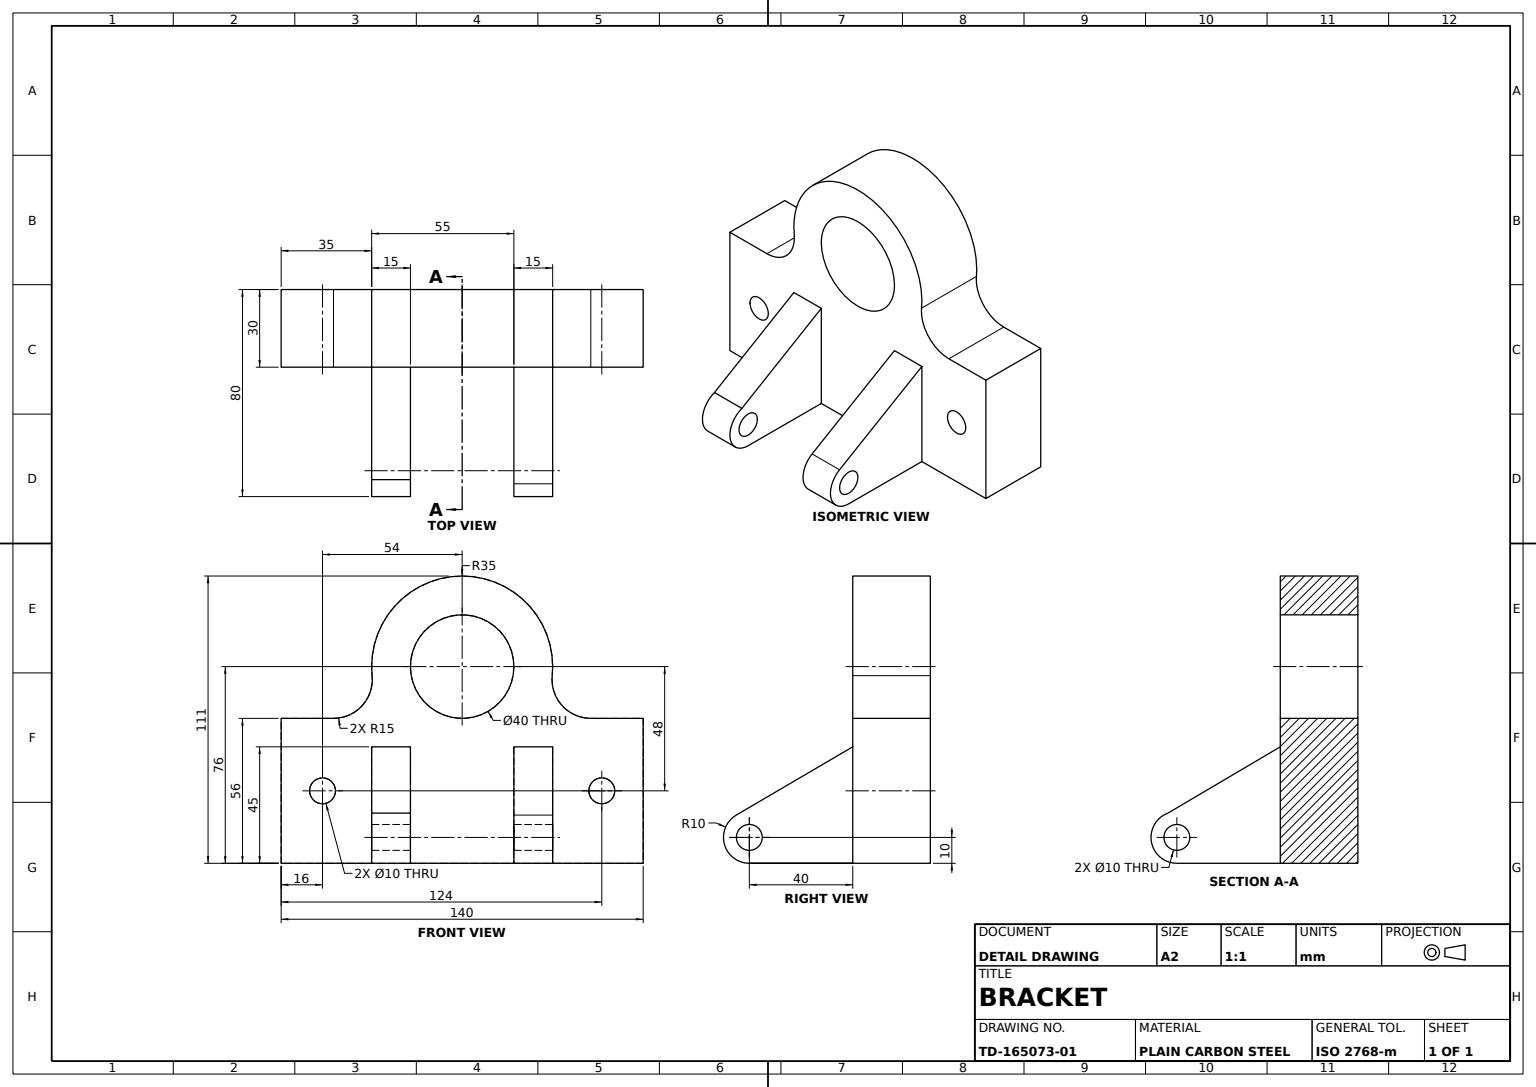
SolidWorks part; units mm, degrees
material "Plain Carbon Steel"
ref_plane "Front Plane" through (0, 0, 0) normal (0, 0, 1) x (1, 0, 0)
ref_plane "Top Plane" through (0, 0, 0) normal (0, 1, 0) x (1, 0, 0)
ref_plane "Right Plane" through (0, 0, 0) normal (1, 0, 0) x (0, 0, -1)
sketch "Base Profile Sketch" plane through (0, 0, 0) normal (1, 0, 0) x (0, 0, -1)
  line L0 (0, 0) -> (-70, 0)
  line L1 (-70, 0) -> (-70, 56)
  line L2 (0, 0) -> (70, 0)
  line L3 (70, 0) -> (70, 56)
  line L5 (-70, 56) -> (-49.7494, 56)
  line L6 (49.7494, 56) -> (70, 56)
  arc A0 (34.8246, 72.5) -> (-34.8246, 72.5) centre (0, 76) ccw
  arc A1 (-49.7494, 56) -> (-34.8246, 72.5) centre (-49.7494, 71) ccw
  arc A2 (34.8246, 72.5) -> (49.7494, 56) centre (49.7494, 71) ccw
  dimension "D1" = 56
  dimension "D4" = 70
  dimension "D5" = 76
  dimension "D6" = 70
  dimension "D7" = 15
  dimension "D8" = 15
  dimension "D2" = 70
  dimension "D3" = 140
extrude "Pillow Block Base" add sketch "Base Profile Sketch" along normal mid plane 30
ref_plane "Lug Arm 1 Plane" through (0, 0, 20) normal (0, 0, 1) x (1, 0, 0)
sketch "Lug Arm 1 Sketch" plane through (0, 0, 20) normal (0, 0, 1) x (1, 0, 0)
  line L0 (15, 0) -> (55, 0)
  line L2 (15, 0) -> (15, 45)
  line L3 (15, 56) -> (15, 0) construction
  line L4 (15, 45) -> (58.4498, 19.3861)
  arc A0 (55, 0) -> (58.4498, 19.3861) centre (55, 10) ccw
  dimension "D1" = 10
  dimension "D3" = 55
  dimension "D2" = 50.4376
  dimension "D4" = 149.48
extrude "Lug Arm 1" add sketch "Lug Arm 1 Sketch" along normal blind 15
ref_plane "Lug Arm 2 Plane" through (0, 0, -20) normal (0, 0, 1) x (1, 0, 0)
sketch "Lug Arm 2 Sketch" plane through (0, 0, -20) normal (0, 0, 1) x (1, 0, 0)
  line L0 (15, 0) -> (55, 0)
  line L2 (60.0515, 18.6303) -> (15, 45)
  line L3 (15, 45) -> (15, 0)
  arc A0 (55, 0) -> (60.0515, 18.6303) centre (55, 10) ccw
extrude "Lug Arm 2" add sketch "Lug Arm 2 Sketch" against normal blind 15
sketch "Lug Pin Hole Sketch" plane through (0, 0, -35) normal (0, 0, -1) x (-1, 0, 0)
  circle A0 centre (-55, 10) radius 5
  dimension "D1" = 10
extrude "Lug Pin Hole" cut sketch "Lug Pin Hole Sketch" against normal blind 100
sketch "Mounting Holes Sketch" plane through (15, 0, 0) normal (1, 0, 0) x (0, 0, -1)
  line L0 (35, 0) -> (70, 0) construction
  line L1 (70, 0) -> (70, 56) construction
  circle A0 centre (-54, 28) radius 5
  circle A1 centre (54, 28) radius 5
  dimension "D1" = 10
  dimension "D2" = 16
  dimension "D3" = 124
  dimension "D4" = 28
extrude "Mounting Holes 2x" cut sketch "Mounting Holes Sketch" against normal blind 100
sketch "Shaft Bore Sketch" plane through (15, 0, 0) normal (1, 0, 0) x (0, 0, -1)
  circle A0 centre (0, 76) radius 20
  dimension "D1" = 40
extrude "Shaft Bore" cut sketch "Shaft Bore Sketch" against normal blind 100
